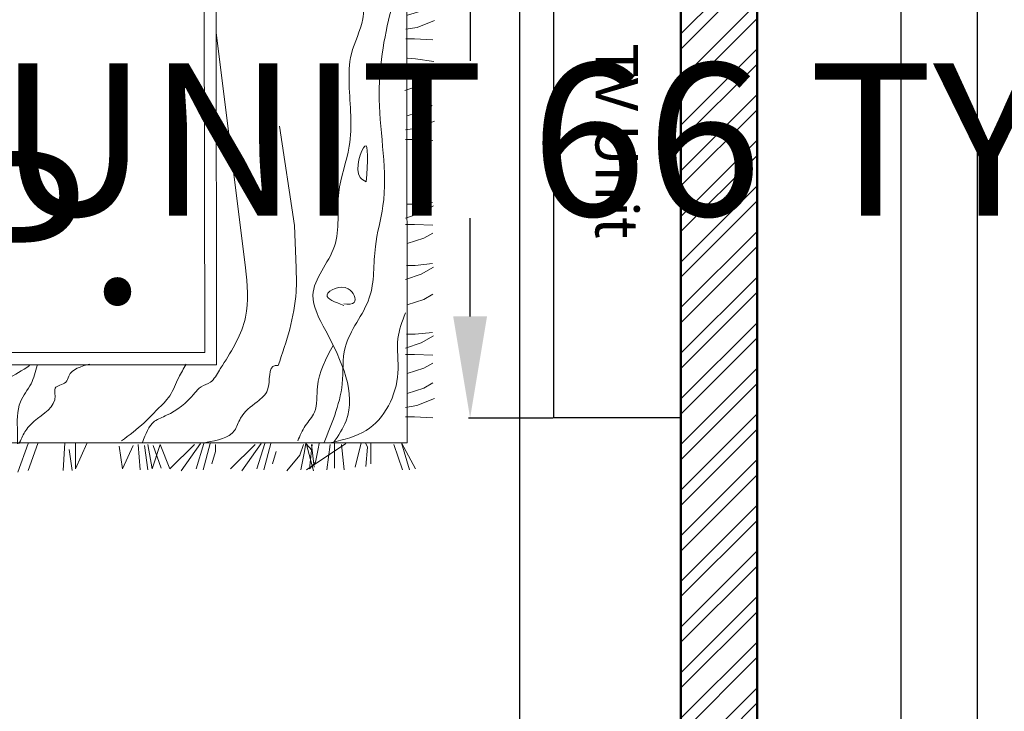
# Model space of a CAD drawing. Units: inches. Extents: x -90 to 536, y -553 to 299.
# Tile 24 of 27: x 294 to 410, y -2 to 80. Entities that reach past the tile are written whole.
import ezdxf

# ---------------------------------------------------------------- set-up
doc = ezdxf.new("R2010")
doc.units = ezdxf.units.IN
for name, color, linetype, lineweight in [('A-ANNO-DIMS', 2, 'Continuous', 18), ('A-ANNO-TEXT', 7, 'Continuous', 18), ('A-FLOR-CASE', 2, 'Continuous', 25), ('A-WALL-PATT', 252, 'Continuous', 13), ('Furniture', 2, 'Continuous', 18), ('Outer Wall', 1, 'Continuous', 50)]:
    doc.layers.add(name, color=color, linetype=linetype, lineweight=lineweight)
doc.styles.get("Standard").update_dxf_attribs({"font": 'arial.ttf'})
doc.dimstyles.get("Standard").update_dxf_attribs({"dimtxt": 18, "dimasz": 12, "dimexe": 0.18, "dimexo": 0.0625, "dimgap": 0.09, "dimtad": 0, "dimtih": 1, "dimtoh": 1, "dimdec": 0, "dimzin": 0, "dimdsep": 46, "dimlunit": 3, "dimtxsty": 'Standard', "dimcen": 0.09, "dimadec": 0, "dimazin": 0, "dimtfac": 1, "dimtdec": 0, "dimtofl": 0, "dimtmove": 0, "dimatfit": 3, "dimfxl": 1, "dimtolj": 1, "dimtzin": 0, "dimarcsym": 0})

# ---------------------------------------------------------------- blocks, each defined once
blk = doc.blocks.new('A$C2B723114')
for p, q in [((0, 2.9047), (2.8274, 2.9047)), ((0, 2.8487), (0, 2.9047)), ((2.8274, 2.9047), (2.8274, 2.8487)), ((0.4243, 2.8697), (0.4243, 2.4855)), ((2.4742, 2.8697), (2.4742, 2.4855)), ((2.8274, 2.8487), (0, 2.8487)), ((0.1012, 2.4649), (0.1012, 2.849)), ((0.1396, 2.5033), (0.1396, 2.849)), ((0.6794, 0.7051), (0.6794, 2.8509)), ((0.7187, 0.7435), (0.7187, 2.8509)), ((2.1776, 2.8509), (2.1776, 0.7454)), ((2.216, 2.8509), (2.216, 0.707)), ((2.6798, 2.5052), (2.6798, 2.8509)), ((2.7182, 2.4668), (2.7182, 2.8509)), ((0.6087, 2.6776), (0.295, 2.6776)), ((2.6586, 2.6776), (2.2821, 2.6776)), ((1.3789, 2.4999), (1.3598, 2.5761)), ((2.0593, 2.4999), (2.0402, 2.5761)), ((0.6766, 2.5033), (0.1396, 2.5033)), ((1.3858, 2.4723), (1.3789, 2.4999)), ((2.0662, 2.4723), (2.0593, 2.4999)), ((2.2188, 2.5052), (2.6798, 2.5052)), ((0.6794, 2.4649), (0.1012, 2.4649)), ((0.7191, 2.47), (2.1778, 2.4719)), ((2.2188, 2.4668), (2.7182, 2.4668)), ((2.1771, 2.3036), (0.718, 2.1685)), ((1.0365, 1.6233), (2.1246, 2.2989)), ((2.2287, 1.6076), (2.2523, 1.5035)), ((2.2726, 1.593), (2.3061, 1.5007)), ((0.5047, 1.5819), (0.5353, 1.4945)), ((0.6174, 1.5819), (0.6232, 1.4916)), ((0.6467, 1.5819), (0.6369, 1.5137)), ((0.6571, 1.4945), (0.6571, 1.5765)), ((2.3067, 1.5881), (2.3373, 1.5007)), ((2.4194, 1.5881), (2.4251, 1.4979)), ((2.4487, 1.5881), (2.4389, 1.5199)), ((2.4591, 1.5007), (2.4591, 1.5828)), ((2.4685, 1.4964), (2.216, 1.5022)), ((0.4269, 0.0884), (0.4269, 1.4945)), ((0.4269, 1.4945), (0.6794, 1.4945)), ((2.4685, 1.4964), (2.4685, 0.0903)), ((2.4685, 1.4044), (2.5491, 1.3861)), ((0.3172, 1.3923), (0.4213, 1.3687)), ((0.3318, 1.3485), (0.4241, 1.3149)), ((2.4596, 1.3659), (2.552, 1.3324)), ((0.3367, 1.3143), (0.4241, 1.2838)), ((2.4645, 1.3318), (2.552, 1.3012)), ((2.4645, 1.2928), (2.5548, 1.2871)), ((2.4645, 1.2635), (2.5328, 1.2733)), ((2.4699, 1.2531), (2.552, 1.2163)), ((2.552, 1.2531), (2.4699, 1.2531)), ((2.5435, 1.2276), (2.4699, 1.2163)), ((2.4699, 1.2163), (2.5463, 1.1823)), ((0.3367, 1.2016), (0.427, 1.1959)), ((0.3367, 1.1724), (0.405, 1.1821)), ((0.4241, 1.162), (0.3421, 1.162)), ((0.3421, 1.162), (0.4241, 1.1252)), ((2.5491, 1.1654), (2.467, 1.1597)), ((2.5463, 1.1455), (2.467, 1.1342)), ((2.5491, 1.1342), (2.4699, 1.1201)), ((2.4699, 1.1201), (2.5491, 1.0946)), ((2.5463, 1.1172), (2.4727, 1.0918)), ((2.5491, 1.0946), (2.4699, 1.0635)), ((2.4699, 1.0635), (2.5491, 0.9842)), ((0.4157, 1.0206), (0.3421, 1.0093)), ((2.4642, 1.0267), (2.552, 0.9644)), ((0.3421, 1.0093), (0.4185, 0.9754)), ((0.4213, 0.9584), (0.3392, 0.9527)), ((2.467, 0.9559), (2.552, 0.9333)), ((2.4699, 0.9785), (2.552, 0.9531)), ((0.4185, 0.9386), (0.3392, 0.9272)), ((0.4213, 0.9272), (0.3421, 0.9131)), ((2.4642, 0.9389), (2.4869, 0.9276)), ((2.4869, 0.9276), (2.5265, 0.9163)), ((0.3421, 0.9131), (0.4213, 0.8876)), ((0.4185, 0.9103), (0.3449, 0.8848)), ((2.5265, 0.9163), (2.5491, 0.9163)), ((0.4213, 0.8876), (0.3421, 0.8565)), ((2.4642, 0.8908), (2.5152, 0.8483)), ((0.3421, 0.8565), (0.4213, 0.7772)), ((2.467, 0.8455), (2.5208, 0.8342)), ((2.5152, 0.8483), (2.5491, 0.837)), ((2.5208, 0.8342), (2.552, 0.8285)), ((2.552, 0.8285), (2.5293, 0.8087)), ((0.3364, 0.8197), (0.4241, 0.7574)), ((2.4699, 0.8172), (2.4925, 0.7974)), ((2.5491, 0.8087), (2.4699, 0.8172)), ((2.4925, 0.7974), (2.535, 0.7889)), ((0.3421, 0.7716), (0.4241, 0.7461)), ((2.5491, 0.7606), (2.467, 0.7719)), ((2.535, 0.7889), (2.552, 0.7861)), ((0.3392, 0.7489), (0.4241, 0.7263)), ((2.1776, 0.7454), (0.7187, 0.7435)), ((2.4727, 0.7464), (2.467, 0.7408)), ((2.552, 0.7464), (2.4727, 0.7464)), ((0.359, 0.7206), (0.3987, 0.7093)), ((0.3987, 0.7093), (0.4213, 0.7093)), ((2.216, 0.707), (0.6794, 0.7051)), ((0.9938, 0.6115), (1.7555, 0.7064)), ((2.467, 0.7153), (2.5491, 0.7238)), ((2.552, 0.7096), (2.467, 0.6842)), ((2.5491, 0.6842), (2.4642, 0.6615)), ((0.3421, 0.6601), (0.4213, 0.5808)), ((2.5491, 0.6672), (2.4755, 0.6587)), ((2.4755, 0.6474), (2.5548, 0.6276)), ((0.3364, 0.6233), (0.4241, 0.561)), ((2.4642, 0.6191), (2.4784, 0.6134)), ((2.4784, 0.6134), (2.5406, 0.6077)), ((2.5406, 0.6077), (2.552, 0.6134)), ((0.3421, 0.5752), (0.4241, 0.5497)), ((2.467, 0.5993), (2.4869, 0.5964)), ((2.4869, 0.5964), (2.552, 0.5964)), ((0.3392, 0.5525), (0.4241, 0.5299)), ((2.467, 0.5313), (2.5491, 0.5596)), ((0.359, 0.5242), (0.3987, 0.5129)), ((2.467, 0.5087), (2.5548, 0.5342)), ((2.5548, 0.5342), (2.4699, 0.4889)), ((0.3364, 0.4785), (0.3874, 0.436)), ((1.4523, 0.5021), (1.1305, 0.4537)), ((1.1305, 0.4537), (0.9938, 0.448)), ((0.4213, 0.415), (0.3364, 0.3923)), ((0.3392, 0.4332), (0.393, 0.4219)), ((0.4241, 0.2868), (0.3392, 0.415)), ((0.3874, 0.436), (0.4213, 0.4247)), ((0.393, 0.4219), (0.4241, 0.4162)), ((0.4241, 0.4162), (0.4015, 0.3964)), ((0.3421, 0.4049), (0.3647, 0.3851)), ((0.4213, 0.3964), (0.3421, 0.4049)), ((0.4213, 0.398), (0.3477, 0.3895)), ((0.3647, 0.3851), (0.4072, 0.3766)), ((2.467, 0.4133), (2.552, 0.4019)), ((2.467, 0.2879), (2.552, 0.4076)), ((0.4072, 0.3766), (0.4241, 0.3738)), ((0.4213, 0.3377), (0.3392, 0.3491)), ((0.4241, 0.3236), (0.3449, 0.3236)), ((2.467, 0.319), (2.5548, 0.3134)), ((0.3392, 0.2925), (0.4213, 0.3009)), ((2.4642, 0.3049), (2.5491, 0.2851)), ((0.3477, 0.2571), (0.427, 0.2373)), ((0.3506, 0.2231), (0.4128, 0.2175)), ((0.4128, 0.2175), (0.4241, 0.2231)), ((2.4699, 0.2491), (2.501, 0.2491)), ((2.501, 0.2491), (2.5491, 0.2547)), ((0.359, 0.2061), (0.4241, 0.2061)), ((2.467, 0.2179), (2.5605, 0.1981)), ((2.467, 0.1981), (2.5491, 0.1613)), ((2.467, 0.184), (2.4982, 0.1755)), ((2.4982, 0.1755), (2.5463, 0.1359)), ((0.3392, 0.1042), (0.4213, 0.1325)), ((2.4699, 0.1302), (2.535, 0.1104)), ((0.3392, 0.0815), (0.427, 0.107)), ((0.427, 0.107), (0.3421, 0.0617)), ((1.5674, 0.0962), (1.5844, 0.0453)), ((1.8568, 0.0962), (1.8738, 0.0453)), ((1.9342, 0.0962), (1.9512, 0.0453)), ((2.2236, 0.0962), (2.2406, 0.0453)), ((2.4642, 0.0991), (2.5378, 0.0877)), ((2.535, 0.1104), (2.5491, 0.0991)), ((2.4685, 0.0903), (0.4269, 0.0884)), ((0.5106, 0.0657), (0.5077, 0.0063)), ((0.5106, 0.094), (0.5106, 0.0657)), ((0.5417, 0.094), (0.5474, 0.0572)), ((0.587, 0.0884), (0.604, 0.0346)), ((0.6512, 0.0884), (0.6682, 0.0346)), ((0.713, 0.0657), (0.7101, 0.0063)), ((0.713, 0.094), (0.713, 0.0657)), ((0.7334, 0.0943), (0.7503, 0.0434)), ((0.7786, 0.0915), (0.7786, 0.0632)), ((0.8739, 0.0884), (0.8908, 0.0346)), ((0.956, 0.0943), (0.973, 0.0434)), ((1.0013, 0.0915), (1.0013, 0.0632)), ((1.072, 0.0884), (1.089, 0.0346)), ((1.1338, 0.0657), (1.131, 0.0063)), ((1.1338, 0.094), (1.1338, 0.0657)), ((1.1542, 0.0943), (1.1712, 0.0434)), ((1.1995, 0.0915), (1.1995, 0.0632)), ((1.4088, 0.0657), (1.406, 0.0063)), ((1.4088, 0.094), (1.4088, 0.0657)), ((1.44, 0.094), (1.4456, 0.0572)), ((1.4853, 0.0884), (1.5023, 0.0346)), ((1.6127, 0.0934), (1.6127, 0.0651)), ((1.6127, 0.0651), (1.6184, 0.0085)), ((1.6297, 0.0849), (1.624, 0.0028)), ((1.6721, 0.0877), (1.6693, 0.0623)), ((1.7344, 0.0651), (1.7316, 0.0057)), ((1.7344, 0.0934), (1.7344, 0.0651)), ((1.7655, 0.0934), (1.7712, 0.0566)), ((1.8108, 0.0877), (1.8278, 0.034)), ((1.9795, 0.0934), (1.9795, 0.0651)), ((1.9795, 0.0651), (1.9852, 0.0085)), ((1.9965, 0.0849), (1.9908, 0.0028)), ((2.039, 0.0877), (2.0361, 0.0623)), ((2.1012, 0.0651), (2.0984, 0.0057)), ((2.1012, 0.0934), (2.1012, 0.0651)), ((2.1324, 0.0934), (2.138, 0.0566)), ((2.1777, 0.0877), (2.1946, 0.034)), ((2.2689, 0.0934), (2.2689, 0.0651)), ((2.2689, 0.0651), (2.2746, 0.0085)), ((2.2859, 0.0849), (2.2802, 0.0028)), ((2.3284, 0.0877), (2.3255, 0.0623)), ((2.3906, 0.0651), (2.3878, 0.0057)), ((2.3906, 0.0934), (2.3906, 0.0651)), ((2.4218, 0.0934), (2.4274, 0.0566)), ((2.467, 0.0877), (2.484, 0.034)), ((2.5378, 0.0877), (2.5463, 0.0821)), ((0.5474, 0.0572), (0.57, 0.0006)), ((0.604, 0.0346), (0.621, 0.0063)), ((0.6682, 0.0346), (0.6851, 0.0063)), ((0.7503, 0.0434), (0.773, 0.0037)), ((0.7786, 0.0632), (0.7843, 0.0066)), ((0.8908, 0.0346), (0.9078, 0.0063)), ((0.973, 0.0434), (0.9957, 0.0037)), ((1.0013, 0.0632), (1.007, 0.0066)), ((1.089, 0.0346), (1.106, 0.0063)), ((1.1712, 0.0434), (1.1939, 0.0037)), ((1.1995, 0.0632), (1.2052, 0.0066)), ((1.4456, 0.0572), (1.4683, 0.0006)), ((1.5023, 0.0346), (1.5192, 0.0082)), ((1.5844, 0.0453), (1.607, 0.0057)), ((1.6693, 0.0623), (1.6608, 0.0028)), ((1.7712, 0.0566), (1.7938, 0)), ((1.8278, 0.034), (1.8448, 0.0057)), ((1.8738, 0.0453), (1.8964, 0.0057)), ((1.9512, 0.0453), (1.9739, 0.0057)), ((2.0361, 0.0623), (2.0276, 0.0028)), ((2.138, 0.0566), (2.1607, 0)), ((2.1946, 0.034), (2.2116, 0.0057)), ((2.2406, 0.0453), (2.2632, 0.0057)), ((2.3255, 0.0623), (2.317, 0.0028)), ((2.4274, 0.0566), (2.4501, 0)), ((2.484, 0.034), (2.501, 0.0057))]:
    blk.add_line(p, q)
for centre, radius in [((0.4243, 2.6776), 0.0821), ((2.4742, 2.6776), 0.0821), ((0.4243, 2.6776), 0.0493), ((2.4742, 2.6776), 0.0493)]:
    blk.add_circle(centre, radius)
for centre, radius, start, end in [((0.8078, 2.821), 0.00214, 160.436, 281.8931), ((0.8088, 2.8207), 0.00315, 111.7883, 160.436), ((0.8162, 2.8021), 0.0232, 94.3025, 111.7883), ((0.8091, 2.8151), 0.00394, 21.9904, 101.8931), ((0.8409, 2.7949), 0.0302, 158.579, 188.1335), ((0.7994, 2.8112), 0.0144, 338.579, 21.9904), ((0.8165, 2.7987), 0.0266, 59.3487, 94.3025), ((0.8554, 2.8643), 0.0497, 239.3487, 264.7408), ((0.9202, 3.5684), 0.7568, 264.7408, 268.0921), ((0.8679, 2.7254), 0.0915, 74.0648, 94.2159), ((0.8679, 2.7254), 0.0915, 53.9136, 74.0648), ((0.9409, 4.189), 1.3777, 268.0921, 270.5757), ((0.86, 2.6097), 0.2158, 62.7604, 69.1397), ((0.9466, 3.6164), 0.8051, 270.5757, 274.8018), ((1.0364, 2.548), 0.2671, 87.4614, 94.8018), ((1.042, 2.6745), 0.1405, 79.8101, 87.4614), ((1.1532, 3.2931), 0.488, 259.8101, 263.9133), ((1.204, 3.7695), 0.9671, 263.9133, 270), ((1.204, 3.4318), 0.6294, 270, 277.5469), ((1.2573, 3.0292), 0.2233, 277.5469, 285.744), ((1.3941, 2.5438), 0.281, 98.4372, 105.744), ((1.3747, 2.6748), 0.1486, 90, 98.4372), ((1.3713, 2.8186), 0.0315, 274.4002, 333.4195), ((1.3747, 2.74), 0.0833, 78.7276, 90), ((1.3886, 2.8099), 0.0121, 333.4195, 78.7276), ((1.4882, 2.821), 0.00214, 160.436, 281.8931), ((1.4892, 2.8207), 0.00315, 111.7883, 160.436), ((1.4966, 2.8021), 0.0232, 94.3025, 111.7883), ((1.4895, 2.8151), 0.00394, 21.9904, 101.8931), ((1.5213, 2.7949), 0.0302, 158.579, 188.1335), ((1.4798, 2.8112), 0.0144, 338.579, 21.9904), ((1.4969, 2.7987), 0.0266, 59.3487, 94.3025), ((1.5358, 2.8643), 0.0497, 239.3487, 264.7408), ((1.6006, 3.5684), 0.7568, 264.7408, 268.0921), ((1.5483, 2.7254), 0.0915, 74.0648, 94.2159), ((1.5483, 2.7254), 0.0915, 53.9136, 74.0648), ((1.6213, 4.189), 1.3777, 268.0921, 270.5757), ((1.5404, 2.6097), 0.2158, 62.7604, 69.1397), ((1.627, 3.6164), 0.8051, 270.5757, 274.8018), ((1.7168, 2.548), 0.2671, 87.4614, 94.8018), ((1.7224, 2.6745), 0.1405, 79.8101, 87.4614), ((1.8336, 3.2931), 0.488, 259.8101, 263.9133), ((1.8844, 3.7695), 0.9671, 263.9133, 270), ((1.8844, 3.4318), 0.6294, 270, 277.5469), ((1.9377, 3.0292), 0.2233, 277.5469, 285.744), ((2.0745, 2.5438), 0.281, 98.4372, 105.744), ((2.0551, 2.6748), 0.1486, 90, 98.4372), ((2.0517, 2.8186), 0.0315, 274.4002, 333.4195), ((2.0551, 2.74), 0.0833, 78.7276, 90), ((2.069, 2.8099), 0.0121, 333.4195, 78.7276), ((1.0356, 2.8227), 0.2268, 188.1335, 192.1095), ((0.635, 2.7368), 0.1829, 7.6809, 12.1095), ((0.8679, 2.7254), 0.0915, 36.1766, 53.9136), ((0.8679, 2.7254), 0.0915, 18.4397, 36.1766), ((0.9263, 2.7386), 0.0708, 51.6114, 62.7604), ((0.7461, 2.511), 0.3611, 46.1885, 51.6114), ((0.8523, 2.6218), 0.2076, 39.0349, 46.1885), ((0.923, 2.7382), 0.4535, 0, 6.2324), ((1.716, 2.8227), 0.2268, 188.1335, 192.1095), ((1.3154, 2.7368), 0.1829, 7.6809, 12.1095), ((1.5483, 2.7254), 0.0915, 36.1766, 53.9136), ((1.5483, 2.7254), 0.0915, 18.4397, 36.1766), ((1.6067, 2.7386), 0.0708, 51.6114, 62.7604), ((1.4265, 2.511), 0.3611, 46.1885, 51.6114), ((1.5327, 2.6218), 0.2076, 39.0349, 46.1885), ((1.6034, 2.7382), 0.4535, 0, 6.2324), ((-0.0181, 2.6487), 0.8418, 3.3687, 7.6809), ((0.9783, 2.7239), 0.0455, 28.3168, 39.0349), ((0.8558, 2.6579), 0.1846, 23.0028, 28.3168), ((0.6623, 2.6487), 0.8418, 3.3687, 7.6809), ((1.6587, 2.7239), 0.0455, 28.3168, 39.0349), ((1.5362, 2.6579), 0.1846, 23.0028, 28.3168), ((1.1884, 2.7382), 0.1881, 350.3156, 0), ((1.8688, 2.7382), 0.1881, 350.3156, 0), ((0.1976, 2.6614), 0.6258, 358.3669, 3.3687), ((0.5722, 2.8434), 0.8132, 347.8016, 350.3156), ((0.878, 2.6614), 0.6258, 358.3669, 3.3687), ((1.2526, 2.8434), 0.8132, 347.8016, 350.3156), ((-0.4351, 2.6794), 1.2587, 356.945, 358.3669), ((1.9648, 2.5659), 0.6074, 171.9949, 177.3351), ((1.6528, 2.6098), 0.2924, 167.8016, 171.9949), ((0.2453, 2.6794), 1.2587, 356.945, 358.3669), ((2.6452, 2.5659), 0.6074, 171.9949, 177.3351), ((2.3332, 2.6098), 0.2924, 167.8016, 171.9949), ((-11.7321, 3.2823), 12.5718, 356.49514, 356.94504), ((-11.0517, 3.2823), 12.5718, 356.49514, 356.94504), ((1.4204, 2.5912), 0.0624, 177.3351, 194.0452), ((2.1008, 2.5912), 0.0624, 177.3351, 194.0452), ((1.4917, 3.1364), 0.681, 244.6889, 246.5156), ((2.1721, 3.1364), 0.681, 244.6889, 246.5156), ((0.5206, 2.5319), 0.2961, 350.0016, 356.4951), ((0.879, 2.3515), 0.1345, 93.574, 102.869), ((0.9376, 1.4146), 1.0732, 90.2865, 93.574), ((0.9586, -2.7845), 5.2724, 89.0296, 90.2865), ((0.9954, -0.6123), 3.0999, 87.3904, 89.0296), ((1.0854, 1.364), 1.1216, 85.3824, 87.3904), ((1.4917, 3.1364), 0.681, 246.5156, 248.3423), ((1.4917, 3.1364), 0.681, 248.3423, 250.572), ((1.4917, 3.1364), 0.681, 250.572, 252.8018), ((1.2975, 2.3514), 0.1345, 83.5659, 101.5586), ((1.3002, 2.3754), 0.1104, 72.6136, 83.5659), ((1.201, 2.5319), 0.2961, 350.0016, 356.4951), ((1.5594, 2.3515), 0.1345, 93.574, 102.869), ((1.618, 1.4146), 1.0732, 90.2865, 93.574), ((1.639, -2.7845), 5.2724, 89.0296, 90.2865), ((1.6758, -0.6123), 3.0999, 87.3904, 89.0296), ((1.7658, 1.364), 1.1216, 85.3824, 87.3904), ((2.1721, 3.1364), 0.681, 246.5156, 248.3423), ((2.1721, 3.1364), 0.681, 248.3423, 250.572), ((2.1721, 3.1364), 0.681, 250.572, 252.8018), ((1.9779, 2.3514), 0.1345, 83.5659, 101.5586), ((1.9806, 2.3754), 0.1104, 72.6136, 83.5659), ((0.8298, 2.4774), 0.0178, 170.0016, 196.6978), ((0.8139, 2.4726), 0.00122, 196.6978, 277.1204), ((0.8041, 2.5514), 0.0807, 277.1204, 286.2212), ((0.8068, 2.5419), 0.0707, 286.2212, 297.2841), ((0.8584, 2.4419), 0.0418, 102.869, 117.2841), ((1.28, 3.7729), 1.2952, 265.3824, 267.2509), ((1.228, 2.691), 0.2121, 267.2509, 281.5586), ((1.3965, 2.6828), 0.2118, 252.6136, 260.5159), ((1.4027, 2.7202), 0.2496, 260.5159, 265.9171), ((1.385, 2.4721), 0.000845, 265.9171, 14.0449), ((1.5102, 2.4774), 0.0178, 170.0016, 196.6978), ((1.4943, 2.4726), 0.00122, 196.6978, 277.1204), ((1.4845, 2.5514), 0.0807, 277.1204, 286.2212), ((1.4872, 2.5419), 0.0707, 286.2212, 297.2841), ((1.5388, 2.4419), 0.0418, 102.869, 117.2841), ((1.9604, 3.7729), 1.2952, 265.3824, 267.2509), ((1.9084, 2.691), 0.2121, 267.2509, 281.5586), ((2.0769, 2.6828), 0.2118, 252.6136, 260.5159), ((2.0831, 2.7202), 0.2496, 260.5159, 265.9171), ((2.0654, 2.4721), 0.000845, 265.9171, 14.0449)]:
    blk.add_arc(centre, radius, start, end)
blk.add_ellipse((0.4962, 1.9132), major_axis=(0.4887, -0.4605), ratio=0.503305, start_param=0.491272, end_param=1.591113)
for points, knots in [([(0.427, 1.4678), (0.4036, 1.4582), (0.3693, 1.4441), (0.3335, 1.4344), (0.3221, 1.4313)], [0, 0, 0, 0, 98.452083, 144.639601, 144.639601, 144.639601, 144.639601]), ([(0.6768, 1.3104), (0.6615, 1.3339), (0.6315, 1.3797), (0.604, 1.4501), (0.5417, 1.4748), (0.5064, 1.4871), (0.4848, 1.4945)], [0, 0, 0, 0, 110.980521, 216.571322, 273.316778, 363.252298, 363.252298, 363.252298, 363.252298]), ([(2.5548, 1.4853), (2.5314, 1.4757), (2.5031, 1.4641), (2.4737, 1.4555), (2.4685, 1.454)], [0, 0, 0, 0, 98.452083, 119.481049, 119.481049, 119.481049, 119.481049]), ([(0.4241, 1.4423), (0.4031, 1.437), (0.3691, 1.4284), (0.3351, 1.4199), (0.3221, 1.4167)], [0, 0, 0, 0, 84.638756, 136.955563, 136.955563, 136.955563, 136.955563]), ([(2.552, 1.4598), (2.5309, 1.4545), (2.5031, 1.4475), (2.4753, 1.4406), (2.4685, 1.4389)], [0, 0, 0, 0, 84.638756, 111.94623, 111.94623, 111.94623, 111.94623]), ([(2.2145, 1.4211), (2.233, 1.4246), (2.2636, 1.4303), (2.2761, 1.3837), (2.3429, 1.3967), (2.3949, 1.3342), (2.4474, 1.3031), (2.4698, 1.2898)], [0, 0, 0, 0, 61.886907, 102.717887, 145.699352, 284.082577, 386.765171, 386.765171, 386.765171, 386.765171]), ([(0.6768, 1.286), (0.6567, 1.2911), (0.6145, 1.3017), (0.5543, 1.3533), (0.4816, 1.349), (0.4362, 1.3493), (0.4233, 1.3493)], [0, 0, 0, 0, 80.250278, 168.388677, 295.908361, 346.663112, 346.663112, 346.663112, 346.663112]), ([(0.4233, 1.3445), (0.4367, 1.3385), (0.464, 1.3264), (0.5129, 1.2848), (0.5456, 1.2161), (0.6131, 1.2349), (0.6142, 1.1913), (0.6642, 1.1806), (0.674, 1.144), (0.6817, 1.1154)], [0, 0, 0, 0, 56.745495, 115.23739, 254.956954, 286.678662, 337.828324, 366.201072, 468.500395, 468.500395, 468.500395, 468.500395]), ([(2.2145, 1.319), (2.2295, 1.319), (2.2678, 1.3192), (2.3288, 1.2705), (2.4143, 1.279), (2.4535, 1.2403), (2.4662, 1.2278)], [0, 0, 0, 0, 57.155505, 146.33427, 287.936209, 355.396728, 355.396728, 355.396728, 355.396728]), ([(2.3573, 1.127), (2.3656, 1.1759), (2.3758, 1.2352), (2.3371, 1.1853), (2.3602, 1.1713), (2.3768, 1.1612)], [0, 0, 0, 0, 107.853607, 130.728419, 189.220329, 189.220329, 189.220329, 189.220329]), ([(2.2182, 1.2059), (2.2419, 1.1958), (2.3116, 1.1659), (2.342, 1.0552), (2.4266, 1.0223), (2.4474, 0.9811), (2.462, 0.9684), (2.4698, 0.9616)], [0, 0, 0, 0, 97.73655, 287.59661, 389.176293, 423.403759, 463.679181, 463.679181, 463.679181, 463.679181]), ([(2.2145, 1.1476), (2.2246, 1.1286), (2.2575, 1.0666), (2.3612, 1.0009), (2.431, 0.9336), (2.4662, 0.8996)], [0, 0, 0, 0, 83.02987, 271.460712, 463.033803, 463.033803, 463.033803, 463.033803]), ([(0.6817, 0.8034), (0.6673, 0.8119), (0.6341, 0.8315), (0.5785, 0.8518), (0.5349, 0.8973), (0.4828, 0.9461), (0.4518, 0.9879), (0.4331, 1.013)], [0, 0, 0, 0, 65.318952, 150.437229, 226.833166, 307.58338, 429.454095, 429.454095, 429.454095, 429.454095]), ([(0.4282, 0.9448), (0.4547, 0.9353), (0.496, 0.9206), (0.5223, 0.8436), (0.5628, 0.7946), (0.6113, 0.7575), (0.6214, 0.7173), (0.6539, 0.7022), (0.672, 0.6897), (0.6768, 0.6864)], [0, 0, 0, 0, 102.299436, 159.044876, 303.717955, 348.579152, 391.138254, 454.581655, 477.456496, 477.456496, 477.456496, 477.456496]), ([(2.2145, 0.823), (2.227, 0.8201), (2.261, 0.8121), (2.261, 0.7401), (2.3352, 0.7659), (2.379, 0.6836), (2.4336, 0.6521), (2.4662, 0.6334)], [0, 0, 0, 0, 46.747668, 127.438174, 179.649794, 280.561838, 429.605131, 429.605131, 429.605131, 429.605131]), ([(0.4282, 0.74), (0.4347, 0.7029), (0.444, 0.6496), (0.5194, 0.6274), (0.555, 0.5807), (0.5975, 0.5243), (0.6789, 0.5415), (0.677, 0.5095), (0.6768, 0.5061)], [0, 0, 0, 0, 130.791737, 187.537266, 286.231946, 353.673191, 460.023761, 472.712403, 472.712403, 472.712403, 472.712403]), ([(2.2218, 0.7246), (2.2595, 0.716), (2.3548, 0.6945), (2.4265, 0.6268), (2.4698, 0.586)], [0, 0, 0, 0, 148.665024, 375.555892, 375.555892, 375.555892, 375.555892]), ([(2.3719, 0.6737), (2.3738, 0.6431), (2.3772, 0.5878), (2.3146, 0.6382), (2.3401, 0.7015), (2.2971, 0.6649), (2.2923, 0.6965), (2.289, 0.7176)], [0, 0, 0, 0, 83.446591, 150.887818, 201.642461, 230.015204, 286.760644, 286.760644, 286.760644, 286.760644]), ([(0.6768, 0.6864), (0.7275, 0.655), (0.8251, 0.5944), (0.9391, 0.606), (0.9938, 0.6115)], [0, 0, 0, 0, 225.995823, 434.686543, 434.686543, 434.686543, 434.686543]), ([(2.2145, 0.5167), (2.1764, 0.5522), (2.1051, 0.6184), (1.9357, 0.5803), (1.9385, 0.6342), (1.9388, 0.6395)], [0, 0, 0, 0, 208.073343, 389.01094, 409.01094, 409.01094, 409.01094, 409.01094]), ([(0.6768, 0.5061), (0.7554, 0.4794), (0.8591, 0.4442), (0.9675, 0.4473), (0.9938, 0.448)], [0, 0, 0, 0, 319.374611, 421.61723, 421.61723, 421.61723, 421.61723]), ([(0.4331, 0.4427), (0.4498, 0.4356), (0.4827, 0.4216), (0.5314, 0.3759), (0.632, 0.3884), (0.6996, 0.3513), (0.7423, 0.3278)], [0, 0, 0, 0, 70.931849, 139.556414, 248.154027, 434.709995, 434.709995, 434.709995, 434.709995]), ([(2.4625, 0.1088), (2.4095, 0.1438), (2.2904, 0.2226), (2.0623, 0.1771), (1.9006, 0.2246), (1.7699, 0.2337), (1.6941, 0.2766), (1.5528, 0.2786), (1.4005, 0.2587), (1.2324, 0.3267), (1.059, 0.2939), (0.9218, 0.426), (0.7359, 0.3204), (0.5586, 0.2391), (0.4502, 0.3116), (0.427, 0.3272)], [0, 0, 0, 0, 239.874704, 538.942419, 850.40885, 893.390315, 1047.998294, 1176.505142, 1437.500972, 1637.333004, 1864.324391, 2089.058767, 2248.736533, 2637.953392, 2744.252142, 2744.252142, 2744.252142, 2744.252142]), ([(1.9771, 0.0962), (1.9286, 0.1117), (1.7864, 0.157), (1.5223, 0.1992), (1.2611, 0.141), (1.0527, 0.2023), (0.8859, 0.1885), (0.76, 0.3042), (0.6211, 0.292), (0.5187, 0.3203), (0.4572, 0.3456), (0.4282, 0.3575)], [0, 0, 0, 0, 198.710624, 582.73994, 1031.873213, 1206.082894, 1423.278209, 1655.952104, 1808.744089, 1945.69963, 2068.229211, 2068.229211, 2068.229211, 2068.229211]), ([(0.8474, 0.0943), (0.82, 0.1047), (0.757, 0.1287), (0.6201, 0.1029), (0.4623, 0.1837), (0.4372, 0.2936), (0.4282, 0.3331)], [0, 0, 0, 0, 112.422038, 258.341957, 533.791494, 688.286079, 688.286079, 688.286079, 688.286079]), ([(0.8718, 0.2941), (0.8821, 0.3221), (0.9041, 0.3814), (0.9523, 0.2773), (0.8733, 0.2454), (0.8757, 0.2798), (0.8766, 0.2941)], [0, 0, 0, 0, 82.720021, 175.094899, 237.579423, 282.440623, 282.440623, 282.440623, 282.440623]), ([(1.2715, 0.221), (1.3344, 0.2172), (1.4529, 0.21), (1.2971, 0.2665), (1.2756, 0.2284), (1.2715, 0.221)], [0, 0, 0, 0, 150.888188, 283.977876, 315.699589, 315.699589, 315.699589, 315.699589])]:
    blk.add_open_spline(points, degree=3, knots=knots)
blk = doc.blocks.new('TV-UNIT')
blk.add_lwpolyline([(15, 65.77), (15, 0), (0, 0), (0, 65.77)], close=True)
blk = doc.blocks.new('*D29')
at = {"layer": 'A-ANNO-DIMS', "color": 0, "lineweight": -2, "transparency": 16777216}
for p, q in [((357.07, 98.65), (347.09, 98.65)), ((347.27, 86.65), (347.27, 75.05)), ((347.27, 44.88), (347.27, 56.48)), ((357.07, 32.88), (347.09, 32.88))]:
    blk.add_line(p, q, dxfattribs=at)
at = {"layer": 'A-ANNO-DIMS', "color": 0, "transparency": 16777216}
for points in [[(345.27, 86.65), (349.27, 86.65), (347.27, 98.65)], [(345.27, 44.88), (349.27, 44.88), (347.27, 32.88)]]:
    blk.add_solid(points, dxfattribs=at)
at = {"layer": 'Defpoints', "color": 0, "transparency": 16777216}
for p in [(347.27, 98.65), (357.13, 98.65), (357.13, 32.88)]:
    blk.add_point(p, dxfattribs=at)
at = {"layer": 'A-ANNO-DIMS', "color": 0, "transparency": 16777216, "insert": (347.27, 65.76), "char_height": 18, "attachment_point": 5}
blk.add_mtext('\\A1;TV UNIT 66 TYP.', dxfattribs=at)
blk = doc.blocks.new('*D33')
at = {"layer": 'A-ANNO-DIMS', "color": 0, "lineweight": -2, "transparency": 16777216}
for p, q in [((173.76, 108.4), (189.77, 108.4)), ((189.59, 96.4), (189.59, 64.83)), ((189.59, 14.45), (189.59, 46.02)), ((173.76, 2.45), (189.77, 2.45))]:
    blk.add_line(p, q, dxfattribs=at)
at = {"layer": 'A-ANNO-DIMS', "color": 0, "transparency": 16777216}
for points in [[(187.59, 96.4), (191.59, 96.4), (189.59, 108.4)], [(187.59, 14.45), (191.59, 14.45), (189.59, 2.45)]]:
    blk.add_solid(points, dxfattribs=at)
at = {"layer": 'Defpoints', "color": 0, "transparency": 16777216}
for p in [(173.7, 108.4), (173.7, 2.45), (189.59, 2.45)]:
    blk.add_point(p, dxfattribs=at)
at = {"layer": 'A-ANNO-DIMS', "color": 0, "transparency": 16777216, "insert": (189.59, 55.42), "char_height": 18, "attachment_point": 5}
blk.add_mtext('\\A1;BED GROUP 106 TYP.', dxfattribs=at)
blk = doc.blocks.new('*D39')
at = {"layer": 'A-ANNO-DIMS', "color": 0, "lineweight": -2, "transparency": 16777216}
for p, q in [((209.07, 134.45), (199.12, 134.45)), ((199.3, 122.45), (199.3, 111.07)), ((199.3, 80.89), (199.3, 92.26)), ((209.07, 68.89), (199.12, 68.89))]:
    blk.add_line(p, q, dxfattribs=at)
at = {"layer": 'A-ANNO-DIMS', "color": 0, "transparency": 16777216}
for points in [[(197.3, 122.45), (201.3, 122.45), (199.3, 134.45)], [(197.3, 80.89), (201.3, 80.89), (199.3, 68.89)]]:
    blk.add_solid(points, dxfattribs=at)
at = {"layer": 'Defpoints', "color": 0, "transparency": 16777216}
for p in [(199.3, 134.45), (209.13, 134.45), (209.13, 68.89)]:
    blk.add_point(p, dxfattribs=at)
at = {"layer": 'A-ANNO-DIMS', "color": 0, "transparency": 16777216, "insert": (199.3, 101.67), "char_height": 18, "attachment_point": 5}
blk.add_mtext('\\A1;WARDROBE 66 TYP.', dxfattribs=at)
blk = doc.blocks.new('*D53')
at = {"layer": 'A-ANNO-DIMS', "color": 0, "lineweight": -2, "transparency": 16777216}
for p, q in [((35.09, 103.75), (35.09, 287.38)), ((47.09, 287.2), (183.7, 287.2)), ((395.13, 287.2), (258.52, 287.2)), ((407.13, -63.49), (407.13, 287.38))]:
    blk.add_line(p, q, dxfattribs=at)
at = {"layer": 'A-ANNO-DIMS', "color": 0, "transparency": 16777216}
for points in [[(47.09, 289.2), (47.09, 285.2), (35.09, 287.2)], [(395.13, 289.2), (395.13, 285.2), (407.13, 287.2)]]:
    blk.add_solid(points, dxfattribs=at)
at = {"layer": 'Defpoints', "color": 0, "transparency": 16777216}
for p in [(407.13, 287.2), (35.09, 103.69), (407.13, -63.55)]:
    blk.add_point(p, dxfattribs=at)
at = {"layer": 'A-ANNO-DIMS', "color": 0, "transparency": 16777216, "insert": (221.11, 287.2), "char_height": 18, "attachment_point": 5}
blk.add_mtext('\\A1;372.04', dxfattribs=at)
blk = doc.blocks.new('*D58')
at = {"layer": 'A-ANNO-DIMS', "color": 0, "lineweight": -2, "transparency": 16777216}
for p, q in [((290.13, -71.49), (290.13, 287.38)), ((302.13, 287.2), (308.6, 287.2)), ((341.13, 287.2), (334.66, 287.2)), ((353.13, -71.49), (353.13, 287.38))]:
    blk.add_line(p, q, dxfattribs=at)
at = {"layer": 'A-ANNO-DIMS', "color": 0, "transparency": 16777216}
for points in [[(302.13, 289.2), (302.13, 285.2), (290.13, 287.2)], [(341.13, 289.2), (341.13, 285.2), (353.13, 287.2)]]:
    blk.add_solid(points, dxfattribs=at)
at = {"layer": 'Defpoints', "color": 0, "transparency": 16777216}
for p in [(353.13, 287.2), (290.13, -71.55), (353.13, -71.55)]:
    blk.add_point(p, dxfattribs=at)
at = {"layer": 'A-ANNO-DIMS', "color": 0, "transparency": 16777216, "insert": (321.63, 287.2), "char_height": 18, "attachment_point": 5}
blk.add_mtext('\\A1;63', dxfattribs=at)
blk = doc.blocks.new('*D59')
at = {"layer": 'A-ANNO-DIMS', "color": 0, "lineweight": -2, "transparency": 16777216}
for p, q in [((341.13174, 287.201217), (329.13174, 287.201217)), ((353.13174, -71.491283), (353.13174, 287.381217)), ((398.13174, -71.491283), (398.13174, 287.381217)), ((410.13174, 287.201217), (422.13174, 287.201217))]:
    blk.add_line(p, q, dxfattribs=at)
at = {"layer": 'A-ANNO-DIMS', "color": 0, "transparency": 16777216}
for points in [[(341.13174, 289.201217), (341.13174, 285.201217), (353.13174, 287.201217)], [(410.13174, 289.201217), (410.13174, 285.201217), (398.13174, 287.201217)]]:
    blk.add_solid(points, dxfattribs=at)
at = {"layer": 'Defpoints', "color": 0, "transparency": 16777216}
for p in [(398.13174, 287.201217), (353.13174, -71.553783), (398.13174, -71.553783)]:
    blk.add_point(p, dxfattribs=at)
at = {"layer": 'A-ANNO-DIMS', "color": 0, "transparency": 16777216, "insert": (375.63174, 287.201217), "char_height": 18, "attachment_point": 5}
blk.add_mtext('\\A1;45', dxfattribs=at)

msp = doc.modelspace()

# ---------------------------------------------------------------- hatches: boundary and pattern name
at = {"layer": 'A-WALL-PATT'}
h = msp.add_hatch(dxfattribs=at)
h.set_pattern_fill('ANSI32', color=256, scale=0.4)
h.set_pattern_definition([(45, (-88.8105, -603.6155), (-2.694077, 2.694077), []), (45, (-87.0145, -603.6155), (-2.694077, 2.694077), [])])
h.paths.add_polyline_path([(285.1317, 246.4462), (131.1317, 246.4462), (131.1317, 237.4462), (285.1317, 237.4462)])
h.paths.add_polyline_path([(122.1317, 237.4462), (113.1317, 237.4462), (113.1317, 152.4462), (122.1317, 152.4462), (122.1317, 166.4704)])
h.paths.add_polyline_path([(303.1317, 237.4462), (294.1317, 237.4462), (294.1317, 152.4462), (303.1317, 152.4462)])
h.paths.add_polyline_path([(47.1317, 91.9277), (38.1317, 91.9277), (38.1317, -6.5538), (77.1317, -6.5538), (77.1317, 2.4462), (70.5655, 2.4462), (47.1317, 2.4462)])
h.paths.add_polyline_path([(83.052, -61.5538), (47.1317, -61.5538), (47.1317, -24.5538), (38.1317, -24.5538), (38.1317, -70.5538), (74.052, -70.5538), (74.052, -223.5538), (38.1317, -223.5538), (38.1317, -503.5538), (92.1317, -503.5538), (92.1317, -437.5538), (191.1317, -437.5538), (191.1317, -428.5538), (83.1317, -428.5538), (83.1317, -494.5538), (47.1317, -494.5538), (47.1317, -232.5538), (83.052, -232.5538), (83.052, -70.5538)])
h.paths.add_polyline_path([(407.1317, -63.5538), (381.1317, -63.5538), (381.1317, 91.9277), (372.1317, 91.9277), (372.1317, 32.8805), (372.1317, -63.5538), (306.5745, -63.5538), (237.1317, -63.5538), (237.1317, -38.5538), (233.1317, -38.5538), (233.1317, -71.5538), (398.1317, -71.5538), (398.1317, -152.5538), (233.1317, -152.5538), (233.1317, -161.5538), (398.1317, -161.5538), (398.1317, -368.5538), (233.1317, -368.5538), (233.1317, -377.5538), (407.1317, -377.5538), (407.1317, -161.5538)])
h.paths.add_polyline_path([(261.1317, -422.5538), (252.1317, -422.5538), (252.1317, -428.5538), (233.1317, -428.5538), (233.1317, -437.5538), (261.1317, -437.5538)])
h.paths.add_polyline_path([(191.1317, -368.5538), (180.1317, -368.5538), (180.1317, -335.5538), (131.5919, -335.5538), (131.5919, -344.5538), (171.1317, -344.5538), (171.1317, -392.5538), (180.1317, -392.5538), (180.1317, -377.5538), (191.1317, -377.5538)], flags=17)
h.paths.add_polyline_path([(180.1317, -223.5538), (152.1317, -223.5538), (152.1317, -227.5538), (176.1317, -227.5538), (176.1317, -335.5538), (180.1317, -335.5538)], flags=17)
h.paths.add_polyline_path([(131.5919, -335.5538), (83.1317, -335.5538), (83.1317, -339.5538), (83.1317, -392.5538), (87.1317, -392.5538), (87.1317, -339.5538), (131.5919, -339.5538)], flags=17)
h.paths.add_polyline_path([(197.1317, 2.4462), (77.1317, 2.4462), (77.1317, -1.5538), (113.1317, -1.5538), (113.1317, -71.5538), (181.1317, -71.5538), (181.1317, -67.5538), (117.1317, -67.5538), (117.1317, -1.5538), (177.1317, -1.5538), (177.1317, -37.5538), (181.1317, -37.5538), (181.1317, -1.5538), (197.1317, -1.5538)])
h.paths.add_polyline_path([(173.1317, 138.4462), (122.1317, 138.4462), (122.1317, 134.4462), (173.1317, 134.4462)])
h.paths.add_polyline_path([(213.1317, 237.4462), (209.1317, 237.4462), (209.1317, 134.4462), (233.1317, 134.4462), (233.1317, 68.8889), (233.1317, -2.5538), (237.1317, -2.5538), (237.1317, 134.4462), (258.1317, 134.4462), (258.1317, 138.4462), (213.1317, 138.4462)])

# ---------------------------------------------------------------- linework, layer by layer
at = {"layer": 'Outer Wall'}
for p, q in [((372.1317, 134.4462), (372.1317, -63.5538)), ((381.1317, 91.9277), (381.1317, -63.5538))]:
    msp.add_line(p, q, dxfattribs=at)

# ---------------------------------------------------------------- block references
at = {"layer": 'A-FLOR-CASE'}
msp.add_blockref('TV-UNIT', (357.1317, 32.8805), dxfattribs=at)
at = {"layer": 'Furniture', "xscale": 36.47664764473289, "yscale": 36.47664764473289, "zscale": 36.47664764473289, "rotation": 89.99999999999999}
msp.add_blockref('A$C2B723114', (343.0864, 14.3799), dxfattribs=at)

# ---------------------------------------------------------------- texts
at = {"layer": 'A-ANNO-TEXT', "insert": (367.0624, 47.9792), "char_height": 5, "attachment_point": 3, "rotation": 270}
msp.add_mtext_dynamic_manual_height_columns('\\pxqc;{\\fTimes New Roman|b0|i0|c0|p18;TV Unit}', width=35.23368, gutter_width=12.5, heights=[0], dxfattribs=at)

# ---------------------------------------------------------------- dimensions: what is measured, and where the dimension line sits
at = {"layer": 'A-ANNO-DIMS'}
for base, p1, p2, override, picture, middle in [((407.1317, 287.2012), (35.0873, 103.6916), (407.1317, -63.5538), {"dimdec": 2, "dimlfac": 1, "dimrnd": 0, "dimzin": 0, "dimdsep": 46, "dimlunit": 2}, '*D53', (221.1095, 287.2012)), ((353.1317, 287.2012), (290.1317, -71.5538), (353.1317, -71.5538), {"dimdec": 0, "dimlfac": 1, "dimrnd": 0, "dimzin": 0, "dimdsep": 46, "dimlunit": 2}, '*D58', (321.6317, 287.2012)), ((398.1317, 287.2012), (353.1317, -71.5538), (398.1317, -71.5538), {"dimdec": 0, "dimlfac": 1, "dimrnd": 0, "dimzin": 0, "dimdsep": 46, "dimlunit": 2}, '*D59', (375.6317, 287.2012))]:
    dim = msp.add_linear_dim(base=base, p1=p1, p2=p2, dimstyle='Standard', override=override, dxfattribs=at)
    dim.commit()
    dim.dimension.update_dxf_attribs({"geometry": picture, "text_midpoint": middle})
for base, p1, p2, angle, text, picture, middle in [((199.2981, 134.4462), (209.1317, 68.8889), (209.1317, 134.4462), 90, 'WARDROBE <> TYP.', '*D39', (199.2981, 101.6676)), ((347.2664, 98.6495), (357.1317, 32.8805), (357.1317, 98.6495), 90, 'TV UNIT <> TYP.', '*D29', (347.2664, 65.765)), ((189.5912, 2.4462), (173.698, 108.4009), (173.698, 2.4462), 270, 'BED GROUP <> TYP.', '*D33', (189.5912, 55.4235))]:
    dim = msp.add_linear_dim(base=base, p1=p1, p2=p2, angle=angle, text=text, dimstyle='Standard', override={"dimdec": 0, "dimlfac": 1, "dimrnd": 0, "dimzin": 0, "dimdsep": 46, "dimlunit": 2}, dxfattribs=at)
    dim.commit()
    dim.dimension.update_dxf_attribs({"geometry": picture, "text_midpoint": middle})

doc.saveas('drawing.dxf')
